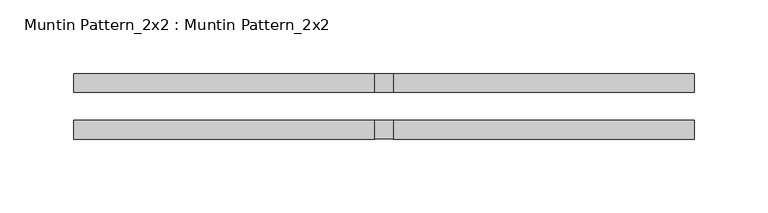
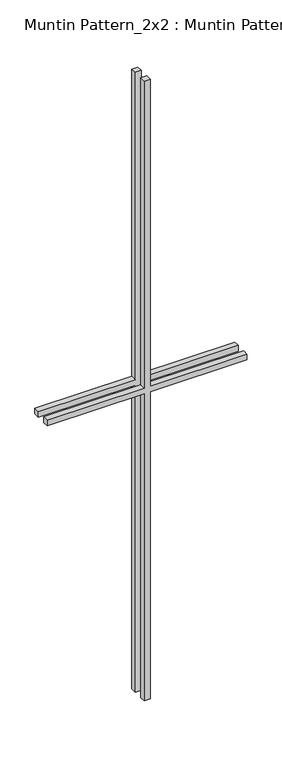
"""IFC4 building model written with IfcOpenShell, lengths in millimetres: proxy geometry, Muntin Pattern_2x2 : Muntin Pattern_2x2."""

from ifc_helpers import new_model, si_unit, frame, origin, place, context, project, spatial, polyline, outline, extrude, source, transform, mapped, element, save


def muntin_pattern_2x2_muntin_pattern_2x2_7b8f790b(model_context):
    return source(origin(), model_context, "Body", "SweptSolid", [
        extrude(outline(polyline([(698.5, -6.35), (698.5, -211.1375), (685.8, -211.1375), (685.8, -6.35), (0.0, -6.35), (0.0, 6.35), (685.8, 6.35), (685.8, 211.1375), (698.5, 211.1375), (698.5, 6.35), (1384.3, 6.35), (1384.3, -6.35), (698.5, -6.35)])), frame((0.0, -22.225, 0.0), z_axis=(0.0, 1.0, 0.0), x_axis=(0.0, 0.0, 1.0)), (0.0, 0.0, 1.0), 12.7),
        extrude(outline(polyline([(698.5, -6.35), (698.5, -211.1375), (685.8, -211.1375), (685.8, -6.35), (0.0, -6.35), (0.0, 6.35), (685.8, 6.35), (685.8, 211.1375), (698.5, 211.1375), (698.5, 6.35), (1384.3, 6.35), (1384.3, -6.35), (698.5, -6.35)])), frame((0.0, 9.525, 0.0), z_axis=(0.0, 1.0, 0.0), x_axis=(0.0, 0.0, 1.0)), (0.0, 0.0, 1.0), 12.7),
    ])


if __name__ == "__main__":
    model = new_model("IFC4")
    model_context = context("Model", 3, world=origin())
    ifc_project = project(units=[si_unit("LENGTHUNIT", "METRE", prefix="MILLI")], contexts=[model_context])
    site = spatial("IfcSite", under=ifc_project)
    building = spatial("IfcBuilding", under=site)
    placement = place(None, origin())
    muntin_pattern_2x2_muntin_pattern_2x2_shape = muntin_pattern_2x2_muntin_pattern_2x2_7b8f790b(model_context)
    element("IfcBuildingElementProxy", 1, Name="Muntin Pattern_2x2 : Muntin Pattern_2x2", ObjectType="Muntin Pattern_2x2 : Muntin Pattern_2x2", at=placement, inside=building, context=model_context, shape_type="MappedRepresentation", body=[
        mapped(muntin_pattern_2x2_muntin_pattern_2x2_shape, transform((0.0, 0.0, 0.0), x_axis=(1.0, 0.0, 0.0), y_axis=(0.0, 1.0, 0.0), z_axis=(0.0, 0.0, 1.0))),
    ])
    save(model, "model.ifc")

# Revit data of these elements
# Type "Muntin Pattern_2x2 : Muntin Pattern_2x2"
#   Width [instance default] = 4' - 0"
#   Thickness = 0' - 0 1/2"
#   Height [instance default] = 4' - 0"
#   Distance = 0' - 0 3/4"
#   Interior Material [instance default] = none
#   Exterior Material [instance default] = none
#   Default Elevation = 0
# Element 1 (IfcBuildingElementProxy, "Muntin Pattern_2x2 : Muntin Pattern_2x2")
#   Width = 1' - 4 5/8"
#   Height = 4' - 6 1/2"
#   Interior Material = Wood - Stained
#   Exterior Material = Clad - White
#   Materials on its faces: "Clad - White", "Wood - Stained"
# Materials
#   "Clad - White": class "Wood", colour RGB 242 242 238, transparency 0, Cost = 0
#   "Wood - Stained": class "Wood", colour RGB 224 178 126, transparency 0, Cost = 0
